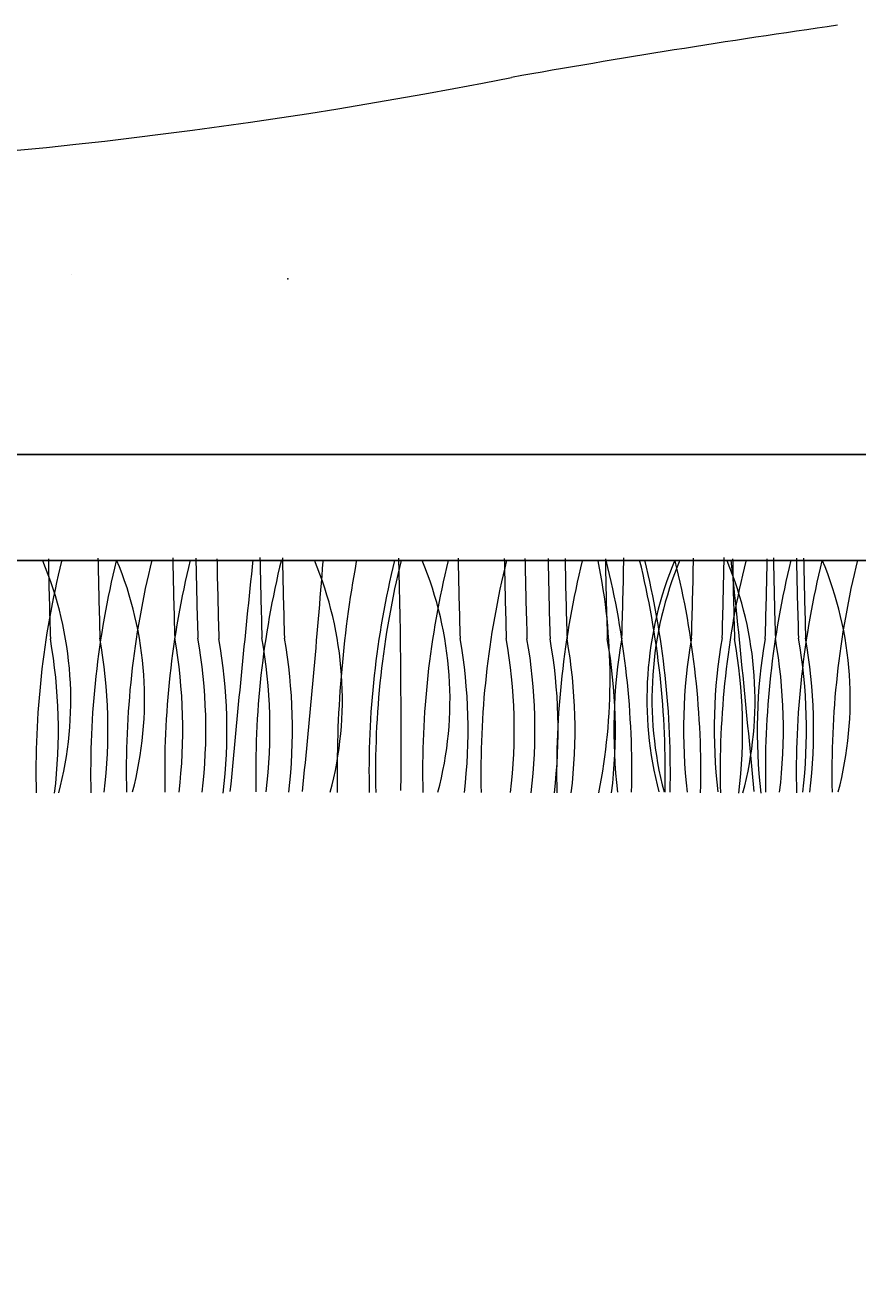
# Model space of a CAD drawing. Units: inches. Extents: x 182 to 1022, y -617 to 111.
# Tile 5 of 33: x 313 to 334, y -309 to -278. Entities that reach past the tile are written whole.
import ezdxf

# ---------------------------------------------------------------- set-up
doc = ezdxf.new("R2010")
doc.units = ezdxf.units.IN
doc.header["$MEASUREMENT"] = 0
doc.layers.add('A-ANNO-DIMS', color=2, linetype='Continuous', lineweight=18)
doc.layers.add('furniture', color=50, linetype='Continuous', lineweight=15, transparency=0.8)
doc.styles.get("Standard").update_dxf_attribs({"font": 'arial.ttf'})
doc.dimstyles.get("Standard").update_dxf_attribs({"dimtxt": 0.18, "dimasz": 0.18, "dimexe": 0.18, "dimexo": 0.0625, "dimgap": 0.09, "dimtad": 0, "dimtih": 1, "dimtoh": 1, "dimdec": 1, "dimzin": 0, "dimdsep": 46, "dimlunit": 4, "dimtxsty": 'Standard', "dimcen": 0.09, "dimadec": 0, "dimazin": 0, "dimtfac": 1, "dimtdec": 1, "dimtofl": 0, "dimtmove": 0, "dimatfit": 3, "dimfxl": 1, "dimtolj": 1, "dimtzin": 0, "dimarcsym": 0})

# ---------------------------------------------------------------- blocks, each defined once
blk = doc.blocks.new('LOUNGE-SEATING-GROUP')
for p, q in [((56.633, 12.696), (56.633, 12.696)), ((134.145, 5.694), (21.664, 5.694)), ((39.442, 5.694), (134.145, 5.694)), ((69.924, 3.919), (69.924, 3.919)), ((70.048, 3.919), (70.048, 3.919)), ((73.886, 3.919), (73.886, 3.919))]:
    blk.add_line(p, q)
for centre, radius, start, end in [((109.316, -219.198), 240.395, 98.11901, 100.04424), ((43.304, 138.877), 123.732, 259.92753, 281.22459), ((77.305, 0.516), 21.554, 166.1427, 181.3669), ((47.768, 2.27), 8.837, 345.1387, 22.6902), ((198.747, 8.279), 142.714, 181.02248, 181.81091), ((78.644, 0.518), 21.554, 166.1427, 181.3669), ((199.961, 8.298), 142.714, 181.02248, 181.81091), ((49.574, 2.293), 8.837, 345.1387, 22.6902), ((79.515, 0.538), 21.554, 166.1427, 181.3669), ((80.456, 0.535), 21.554, 166.1427, 181.3669), ((201.791, 8.299), 142.714, 181.02248, 181.81091), ((202.356, 8.298), 142.714, 181.02248, 181.81091), ((202.872, 8.28), 142.714, 181.02248, 181.81091), ((536.906, -44.164), 478.452, 174.01654, 174.69917), ((82.684, 0.541), 21.554, 166.1427, 181.3669), ((203.925, 8.311), 142.714, 181.02248, 181.81091), ((204.475, 8.303), 142.714, 181.02248, 181.81091), ((-188.034, 25.472), 251.596, 354.19829, 355.48538), ((54.413, 2.289), 8.837, 345.1387, 22.6902), ((91.741, 0.5), 28.62, 169.5961, 180.9805), ((85.455, 0.532), 21.554, 166.1427, 181.3669), ((85.615, 0.531), 21.554, 166.1427, 181.3669), ((-119.833, 1.329), 184.521, 359.60659, 1.37204), ((57.047, 2.285), 8.837, 345.1387, 22.6902), ((86.767, 0.53), 21.554, 166.1427, 181.3669), ((208.773, 8.292), 142.714, 181.02248, 181.81091), ((88.193, 0.526), 21.554, 166.1427, 181.3669), ((209.904, 8.289), 142.714, 181.02248, 181.81091), ((210.41, 8.287), 142.714, 181.02248, 181.81091), ((210.975, 8.286), 142.714, 181.02248, 181.81091), ((90.047, 0.521), 21.554, 166.1427, 181.3669), ((211.39, 8.285), 142.714, 181.02248, 181.81091), ((55.468, 2.803), 14.333, 348.7545, 11.5888), ((212.376, 8.282), 142.714, 181.02248, 181.81091), ((48.78, 0.535), 21.554, 358.6331, 13.8573), ((-72.554, 8.299), 142.714, 358.18909, 358.97752), ((49.597, 0.538), 21.554, 358.6331, 13.8573), ((49.722, 0.538), 21.554, 358.6331, 13.8573), ((79.538, 2.293), 8.837, 157.3098, 194.8613), ((79.662, 2.293), 8.837, 157.3098, 194.8613), ((50.468, 0.518), 21.554, 358.6331, 13.8573), ((-70.849, 8.298), 142.714, 358.18909, 358.97752), ((94.048, 0.516), 21.554, 166.1427, 181.3669), ((-70.099, 8.311), 142.714, 358.18909, 358.97752), ((64.511, 2.27), 8.837, 345.1387, 22.6902), ((-403.08, -44.164), 478.452, 5.30083, 5.98346), ((215.49, 8.279), 142.714, 181.02248, 181.81091), ((-69.046, 8.28), 142.714, 358.18909, 358.97752), ((95.154, 0.535), 21.554, 166.1427, 181.3669), ((216.488, 8.299), 142.714, 181.02248, 181.81091), ((95.911, 0.518), 21.554, 166.1427, 181.3669), ((217.053, 8.298), 142.714, 181.02248, 181.81091), ((217.228, 8.298), 142.714, 181.02248, 181.81091), ((66.841, 2.293), 8.837, 345.1387, 22.6902), ((96.782, 0.538), 21.554, 166.1427, 181.3669), ((43.507, 1.534), 12.794, 353.1171, 10.0651), ((44.721, 1.552), 12.794, 353.1171, 10.0651), ((46.551, 1.553), 12.794, 353.1171, 10.0651), ((47.116, 1.552), 12.794, 353.1171, 10.0651), ((47.632, 1.534), 12.794, 353.1171, 10.0651), ((48.685, 1.565), 12.794, 353.1171, 10.0651), ((49.235, 1.557), 12.794, 353.1171, 10.0651), ((53.533, 1.546), 12.794, 353.1171, 10.0651), ((54.664, 1.543), 12.794, 353.1171, 10.0651), ((55.17, 1.542), 12.794, 353.1171, 10.0651), ((55.735, 1.54), 12.794, 353.1171, 10.0651), ((56.15, 1.539), 12.794, 353.1171, 10.0651), ((57.136, 1.536), 12.794, 353.1171, 10.0651), ((82.686, 1.553), 12.794, 169.9349, 186.8829), ((84.391, 1.552), 12.794, 169.9349, 186.8829), ((85.141, 1.565), 12.794, 169.9349, 186.8829), ((60.25, 1.534), 12.794, 353.1171, 10.0651), ((86.194, 1.534), 12.794, 169.9349, 186.8829), ((61.248, 1.553), 12.794, 353.1171, 10.0651), ((61.813, 1.552), 12.794, 353.1171, 10.0651), ((61.988, 1.552), 12.794, 353.1171, 10.0651)]:
    blk.add_arc(centre, radius, start, end)
blk.add_point((61.918, 12.582))
blk = doc.blocks.new('*D26')
at = {"layer": 'A-ANNO-DIMS', "color": 0, "lineweight": -2, "transparency": 16777216}
for p, q in [((257.848, -296.884), (257.848, -319.733)), ((409.388, -296.884), (409.388, -319.733)), ((258.028, -319.553), (331.642, -319.553)), ((409.208, -319.553), (335.594, -319.553))]:
    blk.add_line(p, q, dxfattribs=at)
at = {"layer": 'A-ANNO-DIMS', "color": 0, "transparency": 16777216}
for points in [[(258.028, -319.523), (258.028, -319.583), (257.848, -319.553)], [(409.208, -319.523), (409.208, -319.583), (409.388, -319.553)]]:
    blk.add_solid(points, dxfattribs=at)
at = {"layer": 'Defpoints', "color": 0, "transparency": 16777216}
for p in [(257.848, -296.822), (409.388, -296.822), (409.388, -319.553)]:
    blk.add_point(p, dxfattribs=at)
at = {"layer": 'A-ANNO-DIMS', "color": 0, "transparency": 16777216, "insert": (333.618, -319.553), "char_height": 0.18, "attachment_point": 5}
blk.add_mtext('\\A1;LOUNGE GROUP 12\'-7 1/2" TYP.', dxfattribs=at)
blk = doc.blocks.new('*D39')
at = {"layer": 'A-ANNO-DIMS', "color": 0, "lineweight": -2, "transparency": 16777216}
for p, q in [((238.398, -288.54), (1015.285, -288.54)), ((1015.105, -288.72), (1015.105, -346.775)), ((1015.105, -405.193), (1015.105, -347.138)), ((238.427, -405.373), (1015.285, -405.373))]:
    blk.add_line(p, q, dxfattribs=at)
at = {"layer": 'A-ANNO-DIMS', "color": 0, "transparency": 16777216}
for points in [[(1015.075, -288.72), (1015.135, -288.72), (1015.105, -288.54)], [(1015.075, -405.193), (1015.135, -405.193), (1015.105, -405.373)]]:
    blk.add_solid(points, dxfattribs=at)
at = {"layer": 'Defpoints', "color": 0, "transparency": 16777216}
for p in [(238.335, -288.54), (1015.105, -288.54), (238.364, -405.373)]:
    blk.add_point(p, dxfattribs=at)
at = {"layer": 'A-ANNO-DIMS', "color": 0, "transparency": 16777216, "insert": (1015.105, -346.956), "char_height": 0.18, "attachment_point": 5}
blk.add_mtext('\\A1;9\'-9"', dxfattribs=at)

msp = doc.modelspace()

# ---------------------------------------------------------------- block references
at = {"layer": 'furniture'}
msp.add_blockref('LOUNGE-SEATING-GROUP', (257.848, -296.822), dxfattribs=at)

# ---------------------------------------------------------------- dimensions: what is measured, and where the dimension line sits
at = {"layer": 'A-ANNO-DIMS'}
dim = msp.add_linear_dim(base=(1015.105, -288.54), p1=(238.364, -405.373), p2=(238.335, -288.54), angle=90, dimstyle='Standard', override={"dimdec": 1, "dimlfac": 1, "dimrnd": 0, "dimzin": 1, "dimdsep": 46, "dimlunit": 4, "dimfrac": 2}, dxfattribs=at)
dim.commit()
dim.dimension.update_dxf_attribs({"geometry": '*D39', "text_midpoint": (1015.105, -346.956)})
dim = msp.add_linear_dim(base=(409.388, -319.553), p1=(257.848, -296.822), p2=(409.388, -296.822), text='LOUNGE GROUP <> TYP.', dimstyle='Standard', override={"dimdec": 1, "dimlfac": 1, "dimrnd": 0, "dimzin": 1, "dimdsep": 46, "dimlunit": 4, "dimfrac": 2}, dxfattribs=at)
dim.commit()
dim.dimension.update_dxf_attribs({"geometry": '*D26', "text_midpoint": (333.618, -319.553)})

doc.saveas('drawing.dxf')
